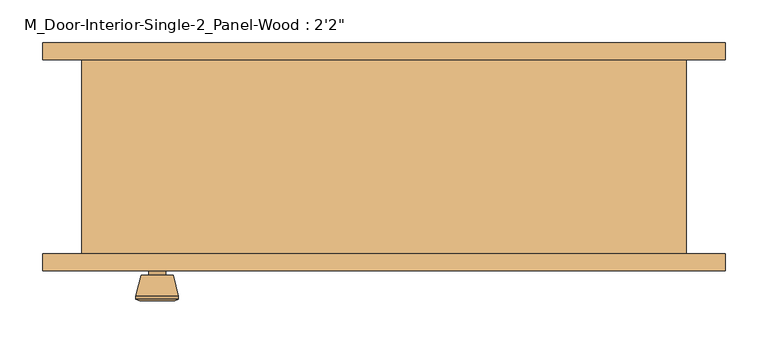
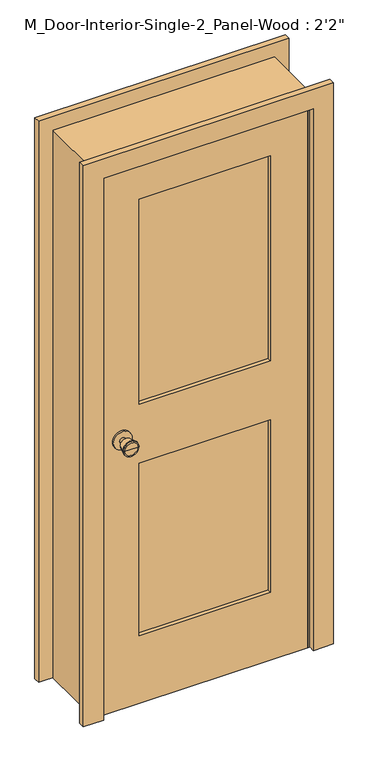
"""IFC4 building model written with IfcOpenShell, lengths in millimetres: door geometry."""

from ifc_helpers import new_model, si_unit, point, frame, frame_2d, origin, place, context, project, spatial, polyline, circle_curve, trimmed, segment, composite_curve, outline, extrude, faceted_brep, source, transform, mapped, element, save
from ifc_brep_helpers import plane_surface, cylinder_surface, revolved_surface, advanced_brep


def door_e2914254(model_context):
    return source(origin(), model_context, "Body", "SolidModel", [
        advanced_brep(
        [(-266.7, -70.125, 914.4), (-276.7, -70.125, 914.4), (-256.7, -70.125, 914.4), (-246.2241324, -21.125, 914.4), (-287.1758676, -21.125, 914.4), (-266.7, -21.125, 914.4), (-241.7, -22.9528681, 914.4), (-291.7, -22.9528681, 914.4), (-241.7, -26.4165463, 914.4), (-291.7, -26.4165463, 914.4), (-248.063764, -51.125, 914.4), (-285.336236, -51.125, 914.4), (-256.7, -51.125, 914.4), (-276.7, -51.125, 914.4)],
        [
            (0, 1),
            (1, 2, circle_curve(frame((-266.7, -70.125, 914.4), z_axis=(0.0, -1.0, 0.0), x_axis=(-1.0, 0.0, 0.0)), 10.0)),
            (2, 0),
            (2, 1, circle_curve(frame((-266.7, -70.125, 914.4), z_axis=(0.0, -1.0, 0.0), x_axis=(-1.0, 0.0, 0.0)), 10.0)),
            (3, 4, circle_curve(frame((-266.7, -21.125, 914.4), z_axis=(0.0, 1.0, 0.0), x_axis=(-1.0, 0.0, 0.0)), 20.4758676)),
            (4, 5),
            (5, 3),
            (4, 3, circle_curve(frame((-266.7, -21.125, 914.4), z_axis=(0.0, 1.0, 0.0), x_axis=(-1.0, 0.0, 0.0)), 20.4758676)),
            (6, 7, circle_curve(frame((-266.7, -22.9528681, 914.4), z_axis=(0.0, 1.0, 0.0), x_axis=(-1.0, 0.0, 0.0)), 25.0)),
            (7, 4),
            (3, 6),
            (7, 6, circle_curve(frame((-266.7, -22.9528681, 914.4), z_axis=(0.0, 1.0, 0.0), x_axis=(-1.0, 0.0, 0.0)), 25.0)),
            (8, 9, circle_curve(frame((-266.7, -26.4165463, 914.4), z_axis=(0.0, 1.0, 0.0), x_axis=(-1.0, 0.0, 0.0)), 25.0)),
            (9, 7),
            (6, 8),
            (9, 8, circle_curve(frame((-266.7, -26.4165463, 914.4), z_axis=(0.0, 1.0, 0.0), x_axis=(-1.0, 0.0, 0.0)), 25.0)),
            (10, 11, circle_curve(frame((-266.7, -51.125, 914.4), z_axis=(0.0, 1.0, 0.0), x_axis=(-1.0, 0.0, 0.0)), 18.636236)),
            (11, 9),
            (8, 10),
            (11, 10, circle_curve(frame((-266.7, -51.125, 914.4), z_axis=(0.0, 1.0, 0.0), x_axis=(-1.0, 0.0, 0.0)), 18.636236)),
            (12, 13, circle_curve(frame((-266.7, -51.125, 914.4), z_axis=(0.0, 1.0, 0.0), x_axis=(-1.0, 0.0, 0.0)), 10.0)),
            (13, 11),
            (10, 12),
            (13, 12, circle_curve(frame((-266.7, -51.125, 914.4), z_axis=(0.0, 1.0, 0.0), x_axis=(-1.0, 0.0, 0.0)), 10.0)),
            (1, 13),
            (12, 2),
        ],
        [
            plane_surface(frame((-266.7, -70.125, 914.4), z_axis=(0.0, -1.0, 0.0), x_axis=(-1.0, 0.0, 0.0))),
            plane_surface(frame((-266.7, -21.125, 914.4), z_axis=(0.0, 1.0, 0.0), x_axis=(-1.0, 0.0, 0.0))),
            revolved_surface(polyline([(-287.1758676, -21.125, 914.4), (-291.7, -22.9528681, 914.4)]), (-266.7, -70.125, 914.4), (0.0, -1.0, 0.0)),
            cylinder_surface(frame((-266.7, -70.125, 914.4), z_axis=(0.0, -1.0, 0.0), x_axis=(-1.0, 0.0, 0.0)), 25.0),
            revolved_surface(polyline([(-291.7, -26.4165463, 914.4), (-285.336236, -51.125, 914.4)]), (-266.7, -70.125, 914.4), (0.0, -1.0, 0.0)),
            plane_surface(frame((-266.7, -51.125, 914.4), z_axis=(0.0, -1.0, 0.0), x_axis=(-1.0, 0.0, 0.0))),
            cylinder_surface(frame((-266.7, -70.125, 914.4), z_axis=(0.0, -1.0, 0.0), x_axis=(-1.0, 0.0, 0.0)), 10.0),
        ],
        [
            (0, [[1, 2, 3]]),
            (0, [[-3, 4, -1]]),
            (1, [[5, 6, 7]]),
            (1, [[8, -7, -6]]),
            (2, [[9, 10, -5, 11]]),
            (2, [[12, -11, -8, -10]]),
            (3, [[13, 14, -9, 15]]),
            (3, [[16, -15, -12, -14]]),
            (4, [[17, 18, -13, 19]]),
            (4, [[20, -19, -16, -18]]),
            (5, [[21, 22, -17, 23]]),
            (5, [[24, -23, -20, -22]]),
            (6, [[-2, 25, -21, 26]]),
            (6, [[-4, -26, -24, -25]]),
        ],
    ),
        extrude(outline(composite_curve([segment(trimmed(circle_curve(frame_2d((914.4, -266.7)), 30.0), [point((914.4, -296.7))], [point((914.4, -236.7))], False, "CARTESIAN"), True, "CONTINUOUS"), segment(trimmed(circle_curve(frame_2d((914.4, -266.7)), 30.0), [point((914.4, -236.7))], [point((914.4, -296.7))], False, "CARTESIAN"), True, "CONTINUOUS")], self_intersect=False)), frame((0.0, -76.125, 0.0), z_axis=(0.0, 1.0, 0.0), x_axis=(0.0, 0.0, 1.0)), (0.0, 0.0, 1.0), 6.0),
        advanced_brep(
        [(-266.7, -117.125, 914.4), (-256.7, -117.125, 914.4), (-276.7, -117.125, 914.4), (-246.2241324, -166.125, 914.4), (-266.7, -166.125, 914.4), (-287.1758676, -166.125, 914.4), (-241.7, -164.2971319, 914.4), (-291.7, -164.2971319, 914.4), (-241.7, -160.8334537, 914.4), (-291.7, -160.8334537, 914.4), (-248.063764, -136.125, 914.4), (-285.336236, -136.125, 914.4), (-256.7, -136.125, 914.4), (-276.7, -136.125, 914.4)],
        [
            (0, 1),
            (1, 2, circle_curve(frame((-266.7, -117.125, 914.4), z_axis=(0.0, 1.0, 0.0), x_axis=(-1.0, 0.0, 0.0)), 10.0)),
            (2, 0),
            (2, 1, circle_curve(frame((-266.7, -117.125, 914.4), z_axis=(0.0, 1.0, 0.0), x_axis=(-1.0, 0.0, 0.0)), 10.0)),
            (3, 4),
            (4, 5),
            (5, 3, circle_curve(frame((-266.7, -166.125, 914.4), z_axis=(0.0, -1.0, 0.0), x_axis=(-1.0, 0.0, 0.0)), 20.4758676)),
            (3, 5, circle_curve(frame((-266.7, -166.125, 914.4), z_axis=(0.0, -1.0, 0.0), x_axis=(-1.0, 0.0, 0.0)), 20.4758676)),
            (6, 3),
            (5, 7),
            (7, 6, circle_curve(frame((-266.7, -164.2971319, 914.4), z_axis=(0.0, -1.0, 0.0), x_axis=(-1.0, 0.0, 0.0)), 25.0)),
            (6, 7, circle_curve(frame((-266.7, -164.2971319, 914.4), z_axis=(0.0, -1.0, 0.0), x_axis=(-1.0, 0.0, 0.0)), 25.0)),
            (8, 6),
            (7, 9),
            (9, 8, circle_curve(frame((-266.7, -160.8334537, 914.4), z_axis=(0.0, -1.0, 0.0), x_axis=(-1.0, 0.0, 0.0)), 25.0)),
            (8, 9, circle_curve(frame((-266.7, -160.8334537, 914.4), z_axis=(0.0, -1.0, 0.0), x_axis=(-1.0, 0.0, 0.0)), 25.0)),
            (10, 8),
            (9, 11),
            (11, 10, circle_curve(frame((-266.7, -136.125, 914.4), z_axis=(0.0, -1.0, 0.0), x_axis=(-1.0, 0.0, 0.0)), 18.636236)),
            (10, 11, circle_curve(frame((-266.7, -136.125, 914.4), z_axis=(0.0, -1.0, 0.0), x_axis=(-1.0, 0.0, 0.0)), 18.636236)),
            (12, 10),
            (11, 13),
            (13, 12, circle_curve(frame((-266.7, -136.125, 914.4), z_axis=(0.0, -1.0, 0.0), x_axis=(-1.0, 0.0, 0.0)), 10.0)),
            (12, 13, circle_curve(frame((-266.7, -136.125, 914.4), z_axis=(0.0, -1.0, 0.0), x_axis=(-1.0, 0.0, 0.0)), 10.0)),
            (1, 12),
            (13, 2),
        ],
        [
            plane_surface(frame((-266.7, -117.125, 914.4), z_axis=(0.0, 1.0, 0.0), x_axis=(-1.0, 0.0, 0.0))),
            plane_surface(frame((-266.7, -166.125, 914.4), z_axis=(0.0, -1.0, 0.0), x_axis=(-1.0, 0.0, 0.0))),
            revolved_surface(polyline([(-287.1758676, -166.125, 914.4), (-291.7, -164.2971319, 914.4)]), (-266.7, -117.125, 914.4), (0.0, 1.0, 0.0)),
            cylinder_surface(frame((-266.7, -117.125, 914.4), z_axis=(0.0, 1.0, 0.0), x_axis=(-1.0, 0.0, 0.0)), 25.0),
            revolved_surface(polyline([(-291.7, -160.8334537, 914.4), (-285.336236, -136.125, 914.4)]), (-266.7, -117.125, 914.4), (0.0, 1.0, 0.0)),
            plane_surface(frame((-266.7, -136.125, 914.4), z_axis=(0.0, 1.0, 0.0), x_axis=(-1.0, 0.0, 0.0))),
            cylinder_surface(frame((-266.7, -117.125, 914.4), z_axis=(0.0, 1.0, 0.0), x_axis=(-1.0, 0.0, 0.0)), 10.0),
        ],
        [
            (0, [[1, 2, 3]]),
            (0, [[-3, 4, -1]]),
            (1, [[5, 6, 7]]),
            (1, [[-6, -5, 8]]),
            (2, [[9, -7, 10, 11]]),
            (2, [[-10, -8, -9, 12]]),
            (3, [[13, -11, 14, 15]]),
            (3, [[-14, -12, -13, 16]]),
            (4, [[17, -15, 18, 19]]),
            (4, [[-18, -16, -17, 20]]),
            (5, [[21, -19, 22, 23]]),
            (5, [[-22, -20, -21, 24]]),
            (6, [[25, -23, 26, -2]]),
            (6, [[-26, -24, -25, -4]]),
        ],
    ),
        extrude(outline(composite_curve([segment(trimmed(circle_curve(frame_2d((914.4, -266.7)), 30.0), [point((914.4, -296.7))], [point((914.4, -236.7))], False, "CARTESIAN"), True, "CONTINUOUS"), segment(trimmed(circle_curve(frame_2d((914.4, -266.7)), 30.0), [point((914.4, -236.7))], [point((914.4, -296.7))], False, "CARTESIAN"), True, "CONTINUOUS")], self_intersect=False)), frame((0.0, -117.125, 0.0), z_axis=(0.0, 1.0, 0.0), x_axis=(0.0, 0.0, 1.0)), (0.0, 0.0, 1.0), 6.0),
        faceted_brep([(355.2, -111.125, 0.0), (330.2, -111.125, 0.0), (330.2, -76.125, 0.0), (317.5, -76.125, 0.0), (317.5, -41.2, 0.0), (330.2, -41.2, 0.0), (330.2, 117.475, 0.0), (355.2, 117.475, 0.0), (355.2, 117.475, 1853.8), (355.2, -111.125, 1853.8), (330.2, 117.475, 1828.8), (-330.2, 117.475, 1828.8), (-330.2, 117.475, 0.0), (-355.2, 117.475, 0.0), (-355.2, 117.475, 1853.8), (330.2, -41.2, 1828.8), (317.5, -41.2, 1816.1), (-317.5, -41.2, 1816.1), (-317.5, -41.2, 0.0), (-330.2, -41.2, 0.0), (-330.2, -41.2, 1828.8), (317.5, -76.125, 1816.1), (330.2, -76.125, 1828.8), (-330.2, -76.125, 1828.8), (-330.2, -76.125, 0.0), (-317.5, -76.125, 0.0), (-317.5, -76.125, 1816.1), (330.2, -111.125, 1828.8), (-355.2, -111.125, 1853.8), (-355.2, -111.125, 0.0), (-330.2, -111.125, 0.0), (-330.2, -111.125, 1828.8)], [[[0, 1, 2, 3, 4, 5, 6, 7]], [[7, 8, 9, 0]], [[6, 10, 11, 12, 13, 14, 8, 7]], [[5, 15, 10, 6]], [[4, 16, 17, 18, 19, 20, 15, 5]], [[3, 21, 16, 4]], [[2, 22, 23, 24, 25, 26, 21, 3]], [[1, 27, 22, 2]], [[0, 9, 28, 29, 30, 31, 27, 1]], [[8, 14, 28, 9]], [[15, 20, 11, 10]], [[21, 26, 17, 16]], [[27, 31, 23, 22]], [[29, 13, 12, 19, 18, 25, 24, 30]], [[14, 13, 29, 28]], [[20, 19, 12, 11]], [[26, 25, 18, 17]], [[31, 30, 24, 23]]]),
        extrude(outline(polyline([(1828.8, -330.2), (0.0, -330.2), (0.0, 330.2), (1828.8, 330.2), (1828.8, -330.2)]), holes=[polyline([(1708.8, -210.2), (1708.8, 210.2), (1014.4, 210.2), (1014.4, -210.2), (1708.8, -210.2)]), polyline([(814.4, -210.2), (814.4, 210.2), (230.0, 210.2), (230.0, -210.2), (814.4, -210.2)])]), frame((0.0, -111.125, 0.0), z_axis=(0.0, 1.0, 0.0), x_axis=(0.0, 0.0, 1.0)), (0.0, 0.0, 1.0), 35.0),
        extrude(outline(polyline([(210.2, -87.7916667), (210.2, -99.4583333), (-210.2, -99.4583333), (-210.2, -87.7916667), (210.2, -87.7916667)])), frame((0.0, 0.0, 1014.4), z_axis=(0.0, 0.0, 1.0), x_axis=(1.0, 0.0, 0.0)), (0.0, 0.0, 1.0), 694.4),
        extrude(outline(polyline([(210.2, -87.7916667), (210.2, -99.4583333), (-210.2, -99.4583333), (-210.2, -87.7916667), (210.2, -87.7916667)])), frame((0.0, 0.0, 230.0), z_axis=(0.0, 0.0, 1.0), x_axis=(1.0, 0.0, 0.0)), (0.0, 0.0, 1.0), 584.4),
        extrude(outline(polyline([(0.0, 401.55), (1900.15, 401.55), (1900.15, -401.55), (0.0, -401.55), (0.0, -336.55), (1835.15, -336.55), (1835.15, 336.55), (0.0, 336.55), (0.0, 401.55)])), frame((0.0, -131.125, 0.0), z_axis=(0.0, 1.0, 0.0), x_axis=(0.0, 0.0, 1.0)), (0.0, 0.0, 1.0), 20.0),
        extrude(outline(polyline([(0.0, 401.55), (1900.15, 401.55), (1900.15, -401.55), (0.0, -401.55), (0.0, -336.55), (1835.15, -336.55), (1835.15, 336.55), (0.0, 336.55), (0.0, 401.55)])), frame((0.0, 117.475, 0.0), z_axis=(0.0, 1.0, 0.0), x_axis=(0.0, 0.0, 1.0)), (0.0, 0.0, 1.0), 20.0),
    ])


if __name__ == "__main__":
    model = new_model("IFC4")
    model_context = context("Model", 3, world=origin())
    ifc_project = project(units=[si_unit("LENGTHUNIT", "METRE", prefix="MILLI")], contexts=[model_context])
    site = spatial("IfcSite", under=ifc_project)
    building = spatial("IfcBuilding", under=site)
    placement = place(None, origin())
    door_shape = door_e2914254(model_context)
    element("IfcDoor", 1, ObjectType="M_Door-Interior-Single-2_Panel-Wood : 2'2\"", at=placement, inside=building, context=model_context, shape_type="MappedRepresentation", body=[
        mapped(door_shape, transform((0.0, 0.0, 0.0), x_axis=(1.0, 0.0, 0.0), y_axis=(0.0, 1.0, 0.0), z_axis=(0.0, 0.0, 1.0))),
    ])
    save(model, "model.ifc")

# Revit data of these elements
# Type "M_Door-Interior-Single-2_Panel-Wood : 2'2\""
#   Type Mark = "11"
#   Assembly Code = "C1020300"
#   Analytic Construction = "Wooden"
#   Top Rail = 0' - 4.72441"
#   Thickness = 0' - 1.37795"
#   Thermal Resistance (R) = 2.5876 (h·ft²·°F)/BTU
#   Swing Angle [instance default] = 90.00°
#   Stiles = 0' - 4.72441"
#   Rough Width = 2' - 3.9685"
#   Rough Height = 6' - 0.98425"
#   Lock Rail = 0' - 7.87402"
#   Height = 6' - 0"
#   Width = 2' - 2"
#   Heat Transfer Coefficient (U) = 0.3865 BTU/(h·ft²·°F)
#   Bottom Rail = 0' - 9.05512"
#   Trim Material = Cherry
#   Panel Material = Cherry
#   Frame Material = Cherry
#   Door Handle Material = Aluminum
#   Visual Light Transmittance = 0
#   Solar Heat Gain Coefficient = 0
#   Wall Closure = (empty or 0)
#   Function = (empty or 0)
# Element 1 (IfcDoor, "M_Door-Interior-Single-2_Panel-Wood : 2'2\"")
#   Materials on its faces: "Cherry", "Aluminum"
# Materials
#   "Cherry": class "Wood", colour RGB 226 177 128, transparency 0, Description = "Prunus Serotina", Cost = 0
#   "Aluminum": class "Metal", colour RGB 247 247 247, transparency 0, Description = "Aluminum 6061", Cost = 0
